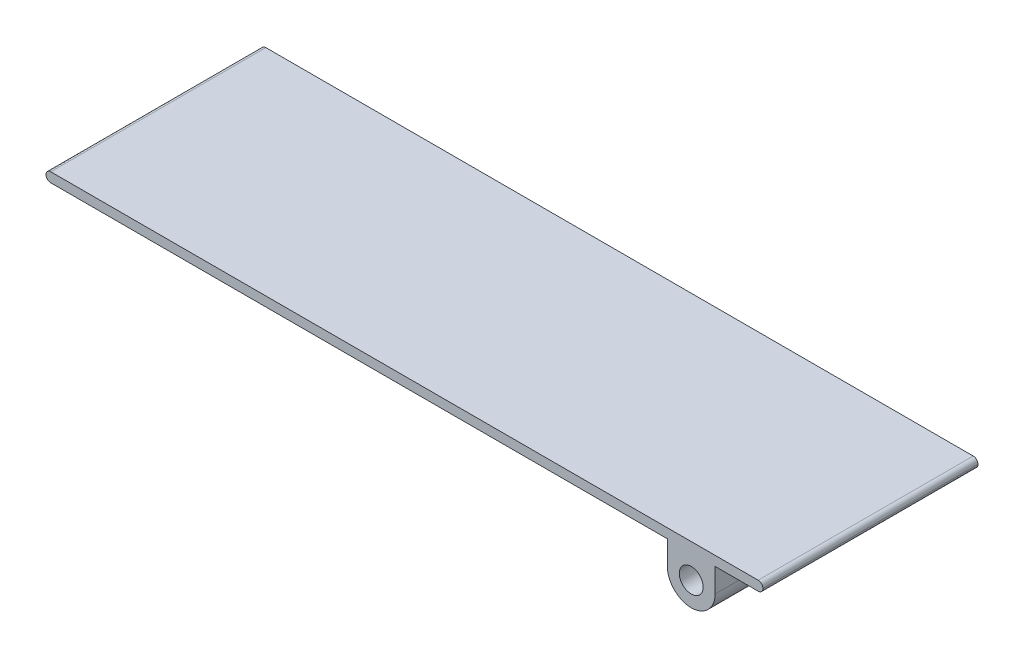
ISO-10303-21;
HEADER;
FILE_DESCRIPTION(('STEP AP214'),'2;1');
FILE_NAME('part.step','',(''),(''),'','','');
FILE_SCHEMA(('AUTOMOTIVE_DESIGN { 1 0 10303 214 1 1 1 1 }'));
ENDSEC;
DATA;
#1=APPLICATION_CONTEXT('core data for automotive mechanical design processes');
#2=APPLICATION_PROTOCOL_DEFINITION('international standard','automotive_design',2000,#1);
#3=PRODUCT_CONTEXT('',#1,'mechanical');
#4=PRODUCT('Part','Part','',(#3));
#5=PRODUCT_RELATED_PRODUCT_CATEGORY('part','',(#4));
#6=PRODUCT_DEFINITION_FORMATION('','',#4);
#7=PRODUCT_DEFINITION_CONTEXT('part definition',#1,'design');
#8=PRODUCT_DEFINITION('design','',#6,#7);
#9=PRODUCT_DEFINITION_SHAPE('','',#8);
#10=(LENGTH_UNIT() NAMED_UNIT(*) SI_UNIT(.MILLI.,.METRE.));
#11=(NAMED_UNIT(*) PLANE_ANGLE_UNIT() SI_UNIT($,.RADIAN.));
#12=(NAMED_UNIT(*) SI_UNIT($,.STERADIAN.) SOLID_ANGLE_UNIT());
#13=UNCERTAINTY_MEASURE_WITH_UNIT(LENGTH_MEASURE(1.E-05),#10,'distance_accuracy_value','');
#14=(GEOMETRIC_REPRESENTATION_CONTEXT(3) GLOBAL_UNCERTAINTY_ASSIGNED_CONTEXT((#13)) GLOBAL_UNIT_ASSIGNED_CONTEXT((#10,
#11,#12)) REPRESENTATION_CONTEXT('',''));
#15=CARTESIAN_POINT('',(0.,0.,0.));
#16=DIRECTION('',(0.,0.,1.));
#17=DIRECTION('',(1.,0.,0.));
#18=AXIS2_PLACEMENT_3D('',#15,#16,#17);
#19=CARTESIAN_POINT('',(0.,-1.,22.5));
#20=DIRECTION('',(0.,1.,0.));
#21=DIRECTION('',(0.,0.,1.));
#22=AXIS2_PLACEMENT_3D('',#19,#20,#21);
#23=PLANE('',#22);
#24=DIRECTION('',(1.,0.,0.));
#25=VECTOR('',#24,1.);
#26=CARTESIAN_POINT('',(0.,-1.,22.5));
#27=LINE('',#26,#25);
#28=CARTESIAN_POINT('',(-74.,-1.,22.5));
#29=VERTEX_POINT('',#28);
#30=CARTESIAN_POINT('',(55.,-1.,22.5));
#31=VERTEX_POINT('',#30);
#32=EDGE_CURVE('E119',#29,#31,#27,.T.);
#33=ORIENTED_EDGE('',*,*,#32,.F.);
#34=DIRECTION('',(0.,0.,-1.));
#35=VECTOR('',#34,1.);
#36=CARTESIAN_POINT('',(-74.,-1.,22.5));
#37=LINE('',#36,#35);
#38=CARTESIAN_POINT('',(-74.,-1.,-22.5));
#39=VERTEX_POINT('',#38);
#40=EDGE_CURVE('E11',#29,#39,#37,.T.);
#41=ORIENTED_EDGE('',*,*,#40,.T.);
#42=DIRECTION('',(1.,0.,0.));
#43=VECTOR('',#42,1.);
#44=CARTESIAN_POINT('',(0.,-1.,-22.5));
#45=LINE('',#44,#43);
#46=CARTESIAN_POINT('',(55.,-1.,-22.5));
#47=VERTEX_POINT('',#46);
#48=EDGE_CURVE('E136',#39,#47,#45,.T.);
#49=ORIENTED_EDGE('',*,*,#48,.T.);
#50=DIRECTION('',(0.,0.,-1.));
#51=VECTOR('',#50,1.);
#52=CARTESIAN_POINT('',(55.,-1.,22.5));
#53=LINE('',#52,#51);
#54=EDGE_CURVE('E134',#31,#47,#53,.T.);
#55=ORIENTED_EDGE('',*,*,#54,.F.);
#56=EDGE_LOOP('',(#33,#41,#49,#55));
#57=FACE_BOUND('',#56,.T.);
#58=ADVANCED_FACE('F41',(#57),#23,.F.);
#59=CARTESIAN_POINT('',(55.,0.,22.5));
#60=DIRECTION('',(1.,0.,0.));
#61=DIRECTION('',(0.,0.,-1.));
#62=AXIS2_PLACEMENT_3D('',#59,#60,#61);
#63=PLANE('',#62);
#64=DIRECTION('',(0.,-1.,0.));
#65=VECTOR('',#64,1.);
#66=CARTESIAN_POINT('',(55.,0.,-22.5));
#67=LINE('',#66,#65);
#68=CARTESIAN_POINT('',(55.,-6.,-22.5));
#69=VERTEX_POINT('',#68);
#70=EDGE_CURVE('E166',#47,#69,#67,.T.);
#71=ORIENTED_EDGE('',*,*,#70,.T.);
#72=DIRECTION('',(0.,0.,-1.));
#73=VECTOR('',#72,1.);
#74=CARTESIAN_POINT('',(55.,-6.,22.5));
#75=LINE('',#74,#73);
#76=CARTESIAN_POINT('',(55.,-6.,22.5));
#77=VERTEX_POINT('',#76);
#78=EDGE_CURVE('E131',#77,#69,#75,.T.);
#79=ORIENTED_EDGE('',*,*,#78,.F.);
#80=DIRECTION('',(0.,-1.,0.));
#81=VECTOR('',#80,1.);
#82=CARTESIAN_POINT('',(55.,0.,22.5));
#83=LINE('',#82,#81);
#84=EDGE_CURVE('E122',#31,#77,#83,.T.);
#85=ORIENTED_EDGE('',*,*,#84,.F.);
#86=ORIENTED_EDGE('',*,*,#54,.T.);
#87=EDGE_LOOP('',(#71,#79,#85,#86));
#88=FACE_BOUND('',#87,.T.);
#89=ADVANCED_FACE('F132',(#88),#63,.F.);
#90=CARTESIAN_POINT('',(60.,-6.,22.5));
#91=DIRECTION('',(0.,0.,-1.));
#92=DIRECTION('',(-1.,0.,0.));
#93=AXIS2_PLACEMENT_3D('',#90,#91,#92);
#94=CYLINDRICAL_SURFACE('',#93,5.);
#95=CARTESIAN_POINT('',(60.,-6.,-22.5));
#96=DIRECTION('',(0.,0.,1.));
#97=DIRECTION('',(1.,0.,0.));
#98=AXIS2_PLACEMENT_3D('',#95,#96,#97);
#99=CIRCLE('',#98,5.);
#100=CARTESIAN_POINT('',(65.,-6.,-22.5));
#101=VERTEX_POINT('',#100);
#102=EDGE_CURVE('E187',#69,#101,#99,.T.);
#103=ORIENTED_EDGE('',*,*,#102,.T.);
#104=DIRECTION('',(0.,0.,-1.));
#105=VECTOR('',#104,1.);
#106=CARTESIAN_POINT('',(65.,-6.,22.5));
#107=LINE('',#106,#105);
#108=CARTESIAN_POINT('',(65.,-6.,22.5));
#109=VERTEX_POINT('',#108);
#110=EDGE_CURVE('E148',#109,#101,#107,.T.);
#111=ORIENTED_EDGE('',*,*,#110,.F.);
#112=CARTESIAN_POINT('',(60.,-6.,22.5));
#113=DIRECTION('',(0.,0.,1.));
#114=DIRECTION('',(1.,0.,0.));
#115=AXIS2_PLACEMENT_3D('',#112,#113,#114);
#116=CIRCLE('',#115,5.);
#117=EDGE_CURVE('E137',#77,#109,#116,.T.);
#118=ORIENTED_EDGE('',*,*,#117,.F.);
#119=ORIENTED_EDGE('',*,*,#78,.T.);
#120=EDGE_LOOP('',(#103,#111,#118,#119));
#121=FACE_BOUND('',#120,.T.);
#122=ADVANCED_FACE('F209',(#121),#94,.T.);
#123=CARTESIAN_POINT('',(65.,0.,22.5));
#124=DIRECTION('',(1.,0.,0.));
#125=DIRECTION('',(0.,0.,-1.));
#126=AXIS2_PLACEMENT_3D('',#123,#124,#125);
#127=PLANE('',#126);
#128=DIRECTION('',(0.,-1.,0.));
#129=VECTOR('',#128,1.);
#130=CARTESIAN_POINT('',(65.,0.,-22.5));
#131=LINE('',#130,#129);
#132=CARTESIAN_POINT('',(65.,-1.,-22.5));
#133=VERTEX_POINT('',#132);
#134=EDGE_CURVE('E190',#133,#101,#131,.T.);
#135=ORIENTED_EDGE('',*,*,#134,.F.);
#136=DIRECTION('',(0.,0.,-1.));
#137=VECTOR('',#136,1.);
#138=CARTESIAN_POINT('',(65.,-1.,22.5));
#139=LINE('',#138,#137);
#140=CARTESIAN_POINT('',(65.,-1.,22.5));
#141=VERTEX_POINT('',#140);
#142=EDGE_CURVE('E199',#141,#133,#139,.T.);
#143=ORIENTED_EDGE('',*,*,#142,.F.);
#144=DIRECTION('',(0.,-1.,0.));
#145=VECTOR('',#144,1.);
#146=CARTESIAN_POINT('',(65.,0.,22.5));
#147=LINE('',#146,#145);
#148=EDGE_CURVE('E208',#141,#109,#147,.T.);
#149=ORIENTED_EDGE('',*,*,#148,.T.);
#150=ORIENTED_EDGE('',*,*,#110,.T.);
#151=EDGE_LOOP('',(#135,#143,#149,#150));
#152=FACE_BOUND('',#151,.T.);
#153=ADVANCED_FACE('F206',(#152),#127,.T.);
#154=CARTESIAN_POINT('',(0.,-1.,22.5));
#155=DIRECTION('',(0.,1.,0.));
#156=DIRECTION('',(0.,0.,1.));
#157=AXIS2_PLACEMENT_3D('',#154,#155,#156);
#158=PLANE('',#157);
#159=DIRECTION('',(1.,0.,0.));
#160=VECTOR('',#159,1.);
#161=CARTESIAN_POINT('',(0.,-1.,-22.5));
#162=LINE('',#161,#160);
#163=CARTESIAN_POINT('',(74.,-1.,-22.5));
#164=VERTEX_POINT('',#163);
#165=EDGE_CURVE('E195',#133,#164,#162,.T.);
#166=ORIENTED_EDGE('',*,*,#165,.T.);
#167=DIRECTION('',(0.,0.,-1.));
#168=VECTOR('',#167,1.);
#169=CARTESIAN_POINT('',(74.,-0.999999999999999,22.5));
#170=LINE('',#169,#168);
#171=CARTESIAN_POINT('',(74.,-1.,22.5));
#172=VERTEX_POINT('',#171);
#173=EDGE_CURVE('E49',#164,#172,#170,.F.);
#174=ORIENTED_EDGE('',*,*,#173,.T.);
#175=DIRECTION('',(1.,0.,0.));
#176=VECTOR('',#175,1.);
#177=CARTESIAN_POINT('',(0.,-1.,22.5));
#178=LINE('',#177,#176);
#179=EDGE_CURVE('E227',#141,#172,#178,.T.);
#180=ORIENTED_EDGE('',*,*,#179,.F.);
#181=ORIENTED_EDGE('',*,*,#142,.T.);
#182=EDGE_LOOP('',(#166,#174,#180,#181));
#183=FACE_BOUND('',#182,.T.);
#184=ADVANCED_FACE('F214',(#183),#158,.F.);
#185=CARTESIAN_POINT('',(0.,1.,22.5));
#186=DIRECTION('',(0.,1.,0.));
#187=DIRECTION('',(0.,0.,1.));
#188=AXIS2_PLACEMENT_3D('',#185,#186,#187);
#189=PLANE('',#188);
#190=DIRECTION('',(1.,0.,0.));
#191=VECTOR('',#190,1.);
#192=CARTESIAN_POINT('',(0.,1.,22.5));
#193=LINE('',#192,#191);
#194=CARTESIAN_POINT('',(-74.,1.,22.5));
#195=VERTEX_POINT('',#194);
#196=CARTESIAN_POINT('',(74.,1.,22.5));
#197=VERTEX_POINT('',#196);
#198=EDGE_CURVE('E225',#195,#197,#193,.T.);
#199=ORIENTED_EDGE('',*,*,#198,.T.);
#200=DIRECTION('',(0.,0.,-1.));
#201=VECTOR('',#200,1.);
#202=CARTESIAN_POINT('',(74.,1.,22.5));
#203=LINE('',#202,#201);
#204=CARTESIAN_POINT('',(74.,1.,-22.5));
#205=VERTEX_POINT('',#204);
#206=EDGE_CURVE('E145',#197,#205,#203,.T.);
#207=ORIENTED_EDGE('',*,*,#206,.T.);
#208=DIRECTION('',(1.,0.,0.));
#209=VECTOR('',#208,1.);
#210=CARTESIAN_POINT('',(0.,1.,-22.5));
#211=LINE('',#210,#209);
#212=CARTESIAN_POINT('',(-74.,1.,-22.5));
#213=VERTEX_POINT('',#212);
#214=EDGE_CURVE('E198',#213,#205,#211,.T.);
#215=ORIENTED_EDGE('',*,*,#214,.F.);
#216=DIRECTION('',(0.,0.,-1.));
#217=VECTOR('',#216,1.);
#218=CARTESIAN_POINT('',(-74.,1.,22.5));
#219=LINE('',#218,#217);
#220=EDGE_CURVE('E143',#213,#195,#219,.F.);
#221=ORIENTED_EDGE('',*,*,#220,.T.);
#222=EDGE_LOOP('',(#199,#207,#215,#221));
#223=FACE_BOUND('',#222,.T.);
#224=ADVANCED_FACE('F221',(#223),#189,.T.);
#225=CARTESIAN_POINT('',(60.,-6.,22.5));
#226=DIRECTION('',(0.,0.,-1.));
#227=DIRECTION('',(-1.,0.,0.));
#228=AXIS2_PLACEMENT_3D('',#225,#226,#227);
#229=CYLINDRICAL_SURFACE('',#228,2.5);
#230=CARTESIAN_POINT('',(60.,-6.,22.5));
#231=DIRECTION('',(0.,0.,1.));
#232=DIRECTION('',(1.,0.,0.));
#233=AXIS2_PLACEMENT_3D('',#230,#231,#232);
#234=CIRCLE('',#233,2.5);
#235=CARTESIAN_POINT('',(57.5,-6.,22.5));
#236=VERTEX_POINT('',#235);
#237=EDGE_CURVE('E203',#236,#236,#234,.T.);
#238=CARTESIAN_POINT('',(60.,-6.,-22.5));
#239=DIRECTION('',(0.,0.,1.));
#240=DIRECTION('',(1.,0.,0.));
#241=AXIS2_PLACEMENT_3D('',#238,#239,#240);
#242=CIRCLE('',#241,2.5);
#243=CARTESIAN_POINT('',(57.5,-6.,-22.5));
#244=VERTEX_POINT('',#243);
#245=EDGE_CURVE('E130',#244,#244,#242,.T.);
#246=CARTESIAN_POINT('',(57.5,-6.,22.5));
#247=CARTESIAN_POINT('',(57.5,-6.,22.03125));
#248=CARTESIAN_POINT('',(57.5,-6.,21.5625));
#249=CARTESIAN_POINT('',(57.5,-6.,20.625));
#250=CARTESIAN_POINT('',(57.5,-6.,20.15625));
#251=CARTESIAN_POINT('',(57.5,-6.,19.21875));
#252=CARTESIAN_POINT('',(57.5,-6.,18.75));
#253=CARTESIAN_POINT('',(57.5,-6.,17.8125));
#254=CARTESIAN_POINT('',(57.5,-6.,17.34375));
#255=CARTESIAN_POINT('',(57.5,-6.,16.40625));
#256=CARTESIAN_POINT('',(57.5,-6.,15.9375));
#257=CARTESIAN_POINT('',(57.5,-6.,15.));
#258=CARTESIAN_POINT('',(57.5,-6.,14.53125));
#259=CARTESIAN_POINT('',(57.5,-6.,13.59375));
#260=CARTESIAN_POINT('',(57.5,-6.,13.125));
#261=CARTESIAN_POINT('',(57.5,-6.,12.1875));
#262=CARTESIAN_POINT('',(57.5,-6.,11.71875));
#263=CARTESIAN_POINT('',(57.5,-6.,10.78125));
#264=CARTESIAN_POINT('',(57.5,-6.,10.3125));
#265=CARTESIAN_POINT('',(57.5,-6.,9.37499999999999));
#266=CARTESIAN_POINT('',(57.5,-6.,8.90625));
#267=CARTESIAN_POINT('',(57.5,-6.,7.96874999999999));
#268=CARTESIAN_POINT('',(57.5,-6.,7.5));
#269=CARTESIAN_POINT('',(57.5,-6.,6.5625));
#270=CARTESIAN_POINT('',(57.5,-6.,6.09374999999999));
#271=CARTESIAN_POINT('',(57.5,-6.,5.15624999999999));
#272=CARTESIAN_POINT('',(57.5,-6.,4.68749999999999));
#273=CARTESIAN_POINT('',(57.5,-6.,3.74999999999999));
#274=CARTESIAN_POINT('',(57.5,-6.,3.28124999999999));
#275=CARTESIAN_POINT('',(57.5,-6.,2.34375));
#276=CARTESIAN_POINT('',(57.5,-6.,1.87499999999999));
#277=CARTESIAN_POINT('',(57.5,-6.,0.937499999999994));
#278=CARTESIAN_POINT('',(57.5,-6.,0.468749999999993));
#279=CARTESIAN_POINT('',(57.5,-6.,-0.468750000000007));
#280=CARTESIAN_POINT('',(57.5,-6.,-0.937500000000008));
#281=CARTESIAN_POINT('',(57.5,-6.,-1.87500000000001));
#282=CARTESIAN_POINT('',(57.5,-6.,-2.34375000000001));
#283=CARTESIAN_POINT('',(57.5,-6.,-3.28125000000001));
#284=CARTESIAN_POINT('',(57.5,-6.,-3.75000000000001));
#285=CARTESIAN_POINT('',(57.5,-6.,-4.68750000000001));
#286=CARTESIAN_POINT('',(57.5,-6.,-5.15625000000001));
#287=CARTESIAN_POINT('',(57.5,-6.,-6.09375000000001));
#288=CARTESIAN_POINT('',(57.5,-6.,-6.56250000000001));
#289=CARTESIAN_POINT('',(57.5,-6.,-7.50000000000001));
#290=CARTESIAN_POINT('',(57.5,-6.,-7.96875000000001));
#291=CARTESIAN_POINT('',(57.5,-6.,-8.90625000000001));
#292=CARTESIAN_POINT('',(57.5,-6.,-9.37500000000001));
#293=CARTESIAN_POINT('',(57.5,-6.,-10.3125));
#294=CARTESIAN_POINT('',(57.5,-6.,-10.78125));
#295=CARTESIAN_POINT('',(57.5,-6.,-11.71875));
#296=CARTESIAN_POINT('',(57.5,-6.,-12.1875));
#297=CARTESIAN_POINT('',(57.5,-6.,-13.125));
#298=CARTESIAN_POINT('',(57.5,-6.,-13.59375));
#299=CARTESIAN_POINT('',(57.5,-6.,-14.53125));
#300=CARTESIAN_POINT('',(57.5,-6.,-15.));
#301=CARTESIAN_POINT('',(57.5,-6.,-15.9375));
#302=CARTESIAN_POINT('',(57.5,-6.,-16.40625));
#303=CARTESIAN_POINT('',(57.5,-6.,-17.34375));
#304=CARTESIAN_POINT('',(57.5,-6.,-17.8125));
#305=CARTESIAN_POINT('',(57.5,-6.,-18.75));
#306=CARTESIAN_POINT('',(57.5,-6.,-19.21875));
#307=CARTESIAN_POINT('',(57.5,-6.,-20.15625));
#308=CARTESIAN_POINT('',(57.5,-6.,-20.625));
#309=CARTESIAN_POINT('',(57.5,-6.,-21.5625));
#310=CARTESIAN_POINT('',(57.5,-6.,-22.03125));
#311=CARTESIAN_POINT('',(57.5,-6.,-22.5));
#312=B_SPLINE_CURVE_WITH_KNOTS('',3,(#246,#247,#248,#249,#250,#251,#252,#253,#254,#255,#256,
#257,#258,#259,#260,#261,#262,#263,#264,#265,#266,#267,#268,#269,#270,#271,#272,#273,#274,#275,
#276,#277,#278,#279,#280,#281,#282,#283,#284,#285,#286,#287,#288,#289,#290,#291,#292,#293,#294,
#295,#296,#297,#298,#299,#300,#301,#302,#303,#304,#305,#306,#307,#308,#309,#310,#311),
.UNSPECIFIED.,.F.,.F.,(4,2,2,2,2,2,2,2,2,2,2,2,2,2,2,2,2,2,2,2,2,2,2,2,2,2,2,2,2,2,2,2,4),(0.,
1.40625,2.8125,4.21875,5.625,7.03125,8.4375,9.84375,11.25,12.65625,14.0625,15.46875,16.875,
18.28125,19.6875,21.09375,22.5,23.90625,25.3125,26.71875,28.125,29.53125,30.9375,32.34375,33.75,
35.15625,36.5625,37.96875,39.375,40.78125,42.1875,43.59375,45.),.UNSPECIFIED.);
#313=EDGE_CURVE('BSEAM231',#236,#244,#312,.T.);
#314=ORIENTED_EDGE('',*,*,#237,.T.);
#315=ORIENTED_EDGE('',*,*,#245,.F.);
#316=ORIENTED_EDGE('',*,*,#313,.T.);
#317=ORIENTED_EDGE('',*,*,#313,.F.);
#318=EDGE_LOOP('',(#314,#316,#315,#317));
#319=FACE_BOUND('',#318,.T.);
#320=ADVANCED_FACE('F231',(#319),#229,.F.);
#321=CARTESIAN_POINT('',(0.,0.,22.5));
#322=DIRECTION('',(0.,0.,1.));
#323=DIRECTION('',(1.,0.,0.));
#324=AXIS2_PLACEMENT_3D('',#321,#322,#323);
#325=PLANE('',#324);
#326=CARTESIAN_POINT('',(74.,0.,22.5));
#327=DIRECTION('',(0.,0.,1.));
#328=DIRECTION('',(1.,0.,0.));
#329=AXIS2_PLACEMENT_3D('',#326,#327,#328);
#330=CIRCLE('',#329,1.);
#331=CARTESIAN_POINT('',(75.,0.,22.5));
#332=VERTEX_POINT('',#331);
#333=EDGE_CURVE('E63',#172,#332,#330,.T.);
#334=ORIENTED_EDGE('',*,*,#333,.T.);
#335=CARTESIAN_POINT('',(74.,0.,22.5));
#336=DIRECTION('',(0.,0.,1.));
#337=DIRECTION('',(1.,0.,0.));
#338=AXIS2_PLACEMENT_3D('',#335,#336,#337);
#339=CIRCLE('',#338,1.);
#340=EDGE_CURVE('E162',#332,#197,#339,.T.);
#341=ORIENTED_EDGE('',*,*,#340,.T.);
#342=ORIENTED_EDGE('',*,*,#198,.F.);
#343=CARTESIAN_POINT('',(-74.,0.,22.5));
#344=DIRECTION('',(0.,0.,1.));
#345=DIRECTION('',(1.,0.,0.));
#346=AXIS2_PLACEMENT_3D('',#343,#344,#345);
#347=CIRCLE('',#346,1.);
#348=CARTESIAN_POINT('',(-75.,0.,22.5));
#349=VERTEX_POINT('',#348);
#350=EDGE_CURVE('E59',#195,#349,#347,.T.);
#351=ORIENTED_EDGE('',*,*,#350,.T.);
#352=CARTESIAN_POINT('',(-74.,0.,22.5));
#353=DIRECTION('',(0.,0.,1.));
#354=DIRECTION('',(1.,0.,0.));
#355=AXIS2_PLACEMENT_3D('',#352,#353,#354);
#356=CIRCLE('',#355,1.);
#357=EDGE_CURVE('E125',#349,#29,#356,.T.);
#358=ORIENTED_EDGE('',*,*,#357,.T.);
#359=ORIENTED_EDGE('',*,*,#32,.T.);
#360=ORIENTED_EDGE('',*,*,#84,.T.);
#361=ORIENTED_EDGE('',*,*,#117,.T.);
#362=ORIENTED_EDGE('',*,*,#148,.F.);
#363=ORIENTED_EDGE('',*,*,#179,.T.);
#364=EDGE_LOOP('',(#334,#341,#342,#351,#358,#359,#360,#361,#362,#363));
#365=FACE_BOUND('',#364,.T.);
#366=ORIENTED_EDGE('',*,*,#237,.F.);
#367=EDGE_LOOP('',(#366));
#368=FACE_BOUND('',#367,.T.);
#369=ADVANCED_FACE('F116',(#365,#368),#325,.T.);
#370=CARTESIAN_POINT('',(0.,0.,-22.5));
#371=DIRECTION('',(0.,0.,1.));
#372=DIRECTION('',(1.,0.,0.));
#373=AXIS2_PLACEMENT_3D('',#370,#371,#372);
#374=PLANE('',#373);
#375=ORIENTED_EDGE('',*,*,#214,.T.);
#376=CARTESIAN_POINT('',(74.,0.,-22.5));
#377=DIRECTION('',(0.,0.,1.));
#378=DIRECTION('',(1.,0.,0.));
#379=AXIS2_PLACEMENT_3D('',#376,#377,#378);
#380=CIRCLE('',#379,1.);
#381=CARTESIAN_POINT('',(75.,0.,-22.5));
#382=VERTEX_POINT('',#381);
#383=EDGE_CURVE('E158',#205,#382,#380,.F.);
#384=ORIENTED_EDGE('',*,*,#383,.T.);
#385=CARTESIAN_POINT('',(74.,0.,-22.5));
#386=DIRECTION('',(0.,0.,1.));
#387=DIRECTION('',(1.,0.,0.));
#388=AXIS2_PLACEMENT_3D('',#385,#386,#387);
#389=CIRCLE('',#388,1.);
#390=EDGE_CURVE('E156',#382,#164,#389,.F.);
#391=ORIENTED_EDGE('',*,*,#390,.T.);
#392=ORIENTED_EDGE('',*,*,#165,.F.);
#393=ORIENTED_EDGE('',*,*,#134,.T.);
#394=ORIENTED_EDGE('',*,*,#102,.F.);
#395=ORIENTED_EDGE('',*,*,#70,.F.);
#396=ORIENTED_EDGE('',*,*,#48,.F.);
#397=CARTESIAN_POINT('',(-74.,0.,-22.5));
#398=DIRECTION('',(0.,0.,1.));
#399=DIRECTION('',(1.,0.,0.));
#400=AXIS2_PLACEMENT_3D('',#397,#398,#399);
#401=CIRCLE('',#400,1.);
#402=CARTESIAN_POINT('',(-75.,0.,-22.5));
#403=VERTEX_POINT('',#402);
#404=EDGE_CURVE('E155',#39,#403,#401,.F.);
#405=ORIENTED_EDGE('',*,*,#404,.T.);
#406=CARTESIAN_POINT('',(-74.,0.,-22.5));
#407=DIRECTION('',(0.,0.,1.));
#408=DIRECTION('',(1.,0.,0.));
#409=AXIS2_PLACEMENT_3D('',#406,#407,#408);
#410=CIRCLE('',#409,1.);
#411=EDGE_CURVE('E152',#403,#213,#410,.F.);
#412=ORIENTED_EDGE('',*,*,#411,.T.);
#413=EDGE_LOOP('',(#375,#384,#391,#392,#393,#394,#395,#396,#405,#412));
#414=FACE_BOUND('',#413,.T.);
#415=ORIENTED_EDGE('',*,*,#245,.T.);
#416=EDGE_LOOP('',(#415));
#417=FACE_BOUND('',#416,.T.);
#418=ADVANCED_FACE('F182',(#414,#417),#374,.F.);
#419=CARTESIAN_POINT('',(74.,0.,22.5));
#420=DIRECTION('',(0.,0.,1.));
#421=DIRECTION('',(1.,0.,0.));
#422=AXIS2_PLACEMENT_3D('',#419,#420,#421);
#423=CYLINDRICAL_SURFACE('',#422,1.);
#424=DIRECTION('',(0.,0.,-1.));
#425=VECTOR('',#424,1.);
#426=CARTESIAN_POINT('',(75.,0.,-22.5));
#427=LINE('',#426,#425);
#428=EDGE_CURVE('E164',#332,#382,#427,.T.);
#429=ORIENTED_EDGE('',*,*,#428,.F.);
#430=ORIENTED_EDGE('',*,*,#333,.F.);
#431=ORIENTED_EDGE('',*,*,#173,.F.);
#432=ORIENTED_EDGE('',*,*,#390,.F.);
#433=EDGE_LOOP('',(#429,#430,#431,#432));
#434=FACE_BOUND('',#433,.T.);
#435=ADVANCED_FACE('F217',(#434),#423,.T.);
#436=CARTESIAN_POINT('',(74.,0.,22.5));
#437=DIRECTION('',(0.,0.,-1.));
#438=DIRECTION('',(-1.,0.,0.));
#439=AXIS2_PLACEMENT_3D('',#436,#437,#438);
#440=CYLINDRICAL_SURFACE('',#439,1.);
#441=ORIENTED_EDGE('',*,*,#340,.F.);
#442=ORIENTED_EDGE('',*,*,#428,.T.);
#443=ORIENTED_EDGE('',*,*,#383,.F.);
#444=ORIENTED_EDGE('',*,*,#206,.F.);
#445=EDGE_LOOP('',(#441,#442,#443,#444));
#446=FACE_BOUND('',#445,.T.);
#447=ADVANCED_FACE('F219',(#446),#440,.T.);
#448=CARTESIAN_POINT('',(-74.,0.,22.5));
#449=DIRECTION('',(0.,0.,-1.));
#450=DIRECTION('',(-1.,0.,0.));
#451=AXIS2_PLACEMENT_3D('',#448,#449,#450);
#452=CYLINDRICAL_SURFACE('',#451,1.);
#453=ORIENTED_EDGE('',*,*,#40,.F.);
#454=ORIENTED_EDGE('',*,*,#357,.F.);
#455=DIRECTION('',(0.,0.,-1.));
#456=VECTOR('',#455,1.);
#457=CARTESIAN_POINT('',(-75.,0.,22.5));
#458=LINE('',#457,#456);
#459=EDGE_CURVE('E44',#403,#349,#458,.F.);
#460=ORIENTED_EDGE('',*,*,#459,.F.);
#461=ORIENTED_EDGE('',*,*,#404,.F.);
#462=EDGE_LOOP('',(#453,#454,#460,#461));
#463=FACE_BOUND('',#462,.T.);
#464=ADVANCED_FACE('F43',(#463),#452,.T.);
#465=CARTESIAN_POINT('',(-74.,0.,22.5));
#466=DIRECTION('',(0.,0.,1.));
#467=DIRECTION('',(1.,0.,0.));
#468=AXIS2_PLACEMENT_3D('',#465,#466,#467);
#469=CYLINDRICAL_SURFACE('',#468,1.);
#470=ORIENTED_EDGE('',*,*,#350,.F.);
#471=ORIENTED_EDGE('',*,*,#220,.F.);
#472=ORIENTED_EDGE('',*,*,#411,.F.);
#473=ORIENTED_EDGE('',*,*,#459,.T.);
#474=EDGE_LOOP('',(#470,#471,#472,#473));
#475=FACE_BOUND('',#474,.T.);
#476=ADVANCED_FACE('F173',(#475),#469,.T.);
#477=CLOSED_SHELL('',(#58,#89,#122,#153,#184,#224,#320,#369,#418,#435,#447,#464,#476));
#478=MANIFOLD_SOLID_BREP('B2',#477);
#479=ADVANCED_BREP_SHAPE_REPRESENTATION('',(#18,#478),#14);
#480=SHAPE_DEFINITION_REPRESENTATION(#9,#479);
ENDSEC;
END-ISO-10303-21;
